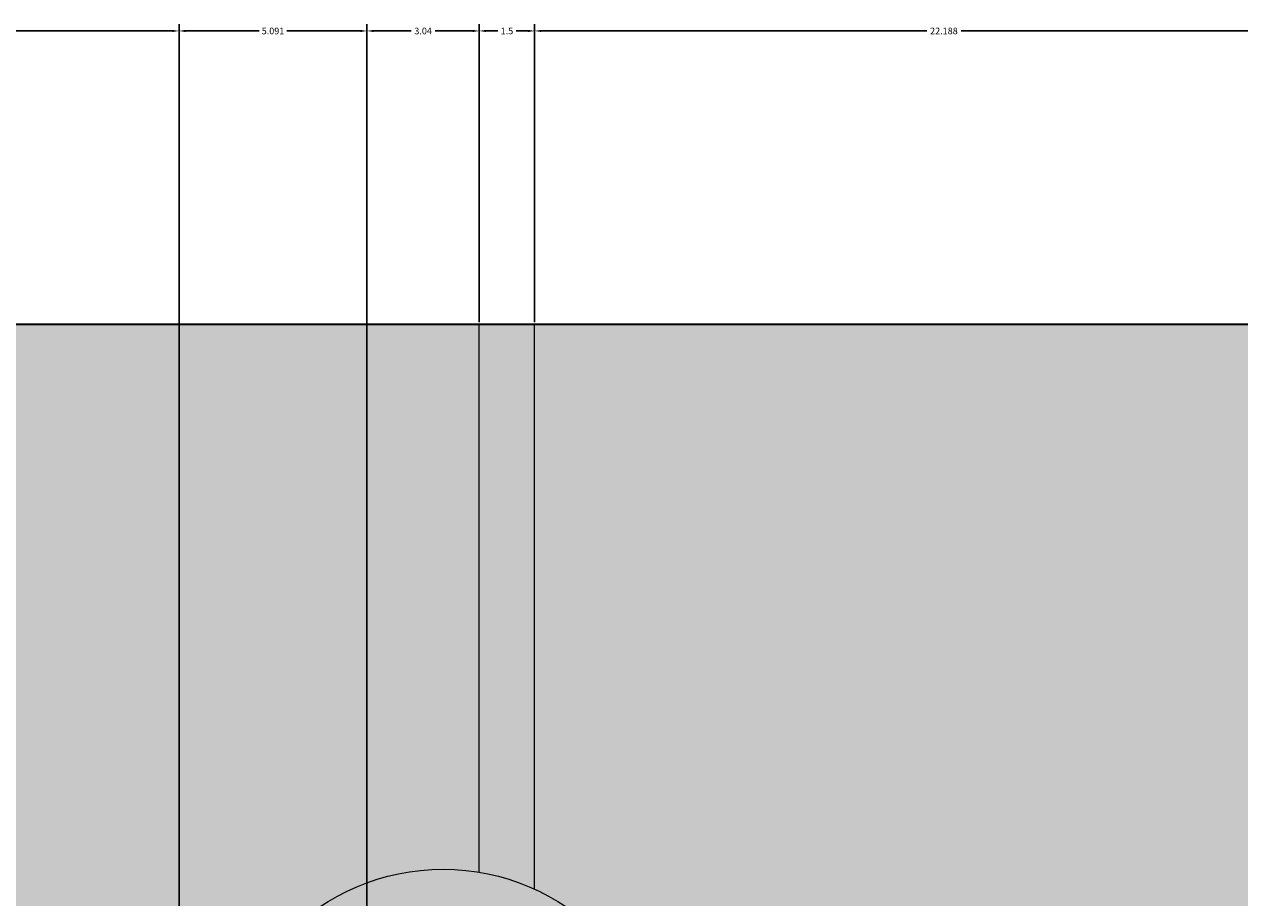
# Model space of a CAD drawing. Units: inches. Extents: x 4508 to 4723, y 847 to 1020.
# Tile 30 of 32: x 4658 to 4691, y 979 to 1003. Entities that reach past the tile are written whole.
import ezdxf

# ---------------------------------------------------------------- set-up
doc = ezdxf.new("R2010")
doc.units = ezdxf.units.IN
for name, color, linetype, lineweight in [('A-ANNO-DIMS', 2, 'Continuous', 18), ('A-WALL', 7, 'Continuous', 35), ('A-WALL-DECO', 6, 'Continuous', 18), ('A-WALL-PATT', 254, 'Continuous', 13)]:
    doc.layers.add(name, color=color, linetype=linetype, lineweight=lineweight)
doc.styles.get("Standard").update_dxf_attribs({"font": 'arial.ttf'})
doc.dimstyles.get("Standard").update_dxf_attribs({"dimtxt": 0.18, "dimasz": 0.18, "dimexe": 0.18, "dimexo": 0.0625, "dimgap": 0.09, "dimtad": 0, "dimtih": 1, "dimtoh": 1, "dimdec": 4, "dimzin": 0, "dimdsep": 46, "dimtxsty": 'Standard', "dimcen": 0.09, "dimadec": 0, "dimazin": 0, "dimtfac": 1, "dimtdec": 4, "dimtofl": 0, "dimtmove": 0, "dimatfit": 3, "dimfxl": 1, "dimtolj": 1, "dimtzin": 0, "dimarcsym": 0})

# ---------------------------------------------------------------- blocks, each defined once
blk = doc.blocks.new('*D7')
at = {"layer": 'A-ANNO-DIMS', "color": 0, "lineweight": -2, "transparency": 16777216}
for p, q in [((4588.994, 994.809), (4588.994, 1002.877)), ((4662.171, 957.665), (4662.171, 1002.877)), ((4589.174, 1002.697), (4625.189, 1002.697)), ((4661.991, 1002.697), (4625.975, 1002.697))]:
    blk.add_line(p, q, dxfattribs=at)
at = {"layer": 'A-ANNO-DIMS', "color": 0, "lineweight": 9, "transparency": 16777216}
for points in [[(4589.174, 1002.727), (4589.174, 1002.667), (4588.994, 1002.697)], [(4661.991, 1002.727), (4661.991, 1002.667), (4662.171, 1002.697)]]:
    blk.add_solid(points, dxfattribs=at)
at = {"layer": 'Defpoints', "color": 0, "lineweight": 9, "transparency": 16777216}
for p in [(4662.171, 1002.697), (4588.994, 994.747), (4662.171, 957.602)]:
    blk.add_point(p, dxfattribs=at)
at = {"layer": 'A-ANNO-DIMS', "color": 0, "transparency": 16777216, "insert": (4625.582, 1002.697), "char_height": 0.18, "attachment_point": 5}
blk.add_mtext('\\A1;73.18', dxfattribs=at)
blk = doc.blocks.new('*D8')
at = {"layer": 'A-ANNO-DIMS', "color": 0, "lineweight": -2, "transparency": 16777216}
for p, q in [((4662.171, 957.665), (4662.171, 1002.877)), ((4667.262, 936.184), (4667.262, 1002.877)), ((4662.351, 1002.697), (4664.34, 1002.697)), ((4667.082, 1002.697), (4665.092, 1002.697))]:
    blk.add_line(p, q, dxfattribs=at)
at = {"layer": 'A-ANNO-DIMS', "color": 0, "lineweight": 9, "transparency": 16777216}
for points in [[(4662.351, 1002.727), (4662.351, 1002.667), (4662.171, 1002.697)], [(4667.082, 1002.727), (4667.082, 1002.667), (4667.262, 1002.697)]]:
    blk.add_solid(points, dxfattribs=at)
at = {"layer": 'Defpoints', "color": 0, "lineweight": 9, "transparency": 16777216}
for p in [(4667.262, 1002.697), (4662.171, 957.602), (4667.262, 936.122)]:
    blk.add_point(p, dxfattribs=at)
at = {"layer": 'A-ANNO-DIMS', "color": 0, "transparency": 16777216, "insert": (4664.716, 1002.697), "char_height": 0.18, "attachment_point": 5}
blk.add_mtext('\\A1;5.091', dxfattribs=at)
blk = doc.blocks.new('*D9')
at = {"layer": 'A-ANNO-DIMS', "color": 0, "lineweight": -2, "transparency": 16777216}
for p, q in [((4667.262, 936.184), (4667.262, 1002.877)), ((4670.306, 994.809), (4670.306, 1002.877)), ((4667.442, 1002.697), (4668.461, 1002.697)), ((4670.126, 1002.697), (4669.107, 1002.697))]:
    blk.add_line(p, q, dxfattribs=at)
at = {"layer": 'A-ANNO-DIMS', "color": 0, "lineweight": 9, "transparency": 16777216}
for points in [[(4667.442, 1002.727), (4667.442, 1002.667), (4667.262, 1002.697)], [(4670.126, 1002.727), (4670.126, 1002.667), (4670.306, 1002.697)]]:
    blk.add_solid(points, dxfattribs=at)
at = {"layer": 'Defpoints', "color": 0, "lineweight": 9, "transparency": 16777216}
for p in [(4670.306, 1002.697), (4670.306, 994.747), (4667.262, 936.122)]:
    blk.add_point(p, dxfattribs=at)
at = {"layer": 'A-ANNO-DIMS', "color": 0, "transparency": 16777216, "insert": (4668.784, 1002.697), "char_height": 0.18, "attachment_point": 5}
blk.add_mtext('\\A1;3.04', dxfattribs=at)
blk = doc.blocks.new('*D10')
at = {"layer": 'A-ANNO-DIMS', "color": 0, "lineweight": -2, "transparency": 16777216}
for p, q in [((4670.306, 994.809), (4670.306, 1002.877)), ((4671.806, 994.809), (4671.806, 1002.877)), ((4670.486, 1002.697), (4670.81, 1002.697)), ((4671.626, 1002.697), (4671.302, 1002.697))]:
    blk.add_line(p, q, dxfattribs=at)
at = {"layer": 'A-ANNO-DIMS', "color": 0, "lineweight": 9, "transparency": 16777216}
for points in [[(4670.486, 1002.727), (4670.486, 1002.667), (4670.306, 1002.697)], [(4671.626, 1002.727), (4671.626, 1002.667), (4671.806, 1002.697)]]:
    blk.add_solid(points, dxfattribs=at)
at = {"layer": 'Defpoints', "color": 0, "lineweight": 9, "transparency": 16777216}
for p in [(4671.806, 1002.697), (4670.306, 994.747), (4671.806, 994.747)]:
    blk.add_point(p, dxfattribs=at)
at = {"layer": 'A-ANNO-DIMS', "color": 0, "transparency": 16777216, "insert": (4671.056, 1002.697), "char_height": 0.18, "attachment_point": 5}
blk.add_mtext('\\A1;1.5', dxfattribs=at)
blk = doc.blocks.new('*D11')
at = {"layer": 'A-ANNO-DIMS', "color": 0, "lineweight": -2, "transparency": 16777216}
for p, q in [((4671.806, 994.809), (4671.806, 1002.877)), ((4693.994, 994.809), (4693.994, 1002.877)), ((4671.986, 1002.697), (4682.435, 1002.697)), ((4693.814, 1002.697), (4683.365, 1002.697))]:
    blk.add_line(p, q, dxfattribs=at)
at = {"layer": 'A-ANNO-DIMS', "color": 0, "lineweight": 9, "transparency": 16777216}
for points in [[(4671.986, 1002.727), (4671.986, 1002.667), (4671.806, 1002.697)], [(4693.814, 1002.727), (4693.814, 1002.667), (4693.994, 1002.697)]]:
    blk.add_solid(points, dxfattribs=at)
at = {"layer": 'Defpoints', "color": 0, "lineweight": 9, "transparency": 16777216}
for p in [(4693.994, 1002.697), (4671.806, 994.747), (4693.994, 994.747)]:
    blk.add_point(p, dxfattribs=at)
at = {"layer": 'A-ANNO-DIMS', "color": 0, "transparency": 16777216, "insert": (4682.9, 1002.697), "char_height": 0.18, "attachment_point": 5}
blk.add_mtext('\\A1;22.188', dxfattribs=at)
blk = doc.blocks.new('*D23')
at = {"layer": 'A-ANNO-DIMS', "color": 0, "lineweight": -2, "transparency": 16777216}
for p, q in [((4694.056, 994.747), (4702.124, 994.747)), ((4701.944, 994.567), (4701.944, 984.545)), ((4701.944, 974.158), (4701.944, 984.181)), ((4669.387, 973.978), (4702.124, 973.978))]:
    blk.add_line(p, q, dxfattribs=at)
at = {"layer": 'A-ANNO-DIMS', "color": 0, "lineweight": 9, "transparency": 16777216}
for points in [[(4701.914, 994.567), (4701.974, 994.567), (4701.944, 994.747)], [(4701.914, 974.158), (4701.974, 974.158), (4701.944, 973.978)]]:
    blk.add_solid(points, dxfattribs=at)
at = {"layer": 'Defpoints', "color": 0, "lineweight": 9, "transparency": 16777216}
for p in [(4693.994, 994.747), (4701.944, 994.747), (4669.325, 973.978)]:
    blk.add_point(p, dxfattribs=at)
at = {"layer": 'A-ANNO-DIMS', "color": 0, "transparency": 16777216, "insert": (4701.944, 984.363), "char_height": 0.18, "attachment_point": 5}
blk.add_mtext('\\A1;20.77', dxfattribs=at)

msp = doc.modelspace()

# ---------------------------------------------------------------- hatches: boundary and pattern name
at = {"layer": 'A-WALL-PATT', "transparency": 33554508}
h = msp.add_hatch(color=256, dxfattribs=at)
h.dxf.hatch_style = 1
h.paths.add_polyline_path([(4661.6706, 954.043, -0.3739004), (4658.5765, 957.6021, -1), (4665.7646, 957.6021, -0.3739004), (4662.6706, 954.043), (4662.6706, 944.4021, -0.2114781), (4670.3062, 945.0869), (4670.3062, 968.0592, -0.4632086), (4663.3246, 973.9783, -0.4632086), (4670.3062, 979.8975), (4670.3062, 994.7469), (4588.9938, 994.7469), (4588.9938, 904.7469), (4657.9938, 904.7469), (4657.9938, 886.7469), (4549.9938, 886.7469), (4549.9938, 878.7469), (4693.9938, 878.7469), (4693.9938, 994.7469), (4671.8062, 994.7469), (4671.8062, 979.4411, -0.2941682), (4675.3246, 973.9783, -0.2941682), (4671.8062, 968.5156), (4671.8062, 944.4278, -0.2741114), (4676.7298, 936.1217, -0.2741114), (4671.8062, 927.8155), (4671.8062, 907.6998, -0.3779645), (4677.0562, 901.7469, -0.3779645), (4671.8062, 895.7939), (4671.8062, 883.7469), (4670.3062, 883.7469), (4670.3062, 895.7939, -0.3779645), (4665.0562, 901.7469, -0.3779645), (4670.3062, 907.6998), (4670.3062, 927.1564, -0.2114781), (4662.6706, 927.8412), (4662.6706, 918.2003, -0.3739004), (4665.7646, 914.6412, -1), (4658.5765, 914.6412, -0.3739004), (4661.6706, 918.2003), (4661.6706, 928.4807, -0.2391825), (4657.7936, 936.1217, -0.2391825), (4661.6706, 943.7626)])
at = {"layer": 'A-WALL-PATT', "transparency": 33554681}
h = msp.add_hatch(color=256, dxfattribs=at)
h.dxf.hatch_style = 1
h.paths.add_polyline_path([(4671.8062, 968.5156, -0.0656104), (4670.3062, 968.0592), (4670.3062, 945.0869, -0.0433429), (4671.8062, 944.4278)])
h.paths.add_polyline_path([(4662.6706, 954.043, -0.0698991), (4661.6706, 954.043), (4661.6706, 943.7626, -0.0313734), (4662.6706, 944.4021)])
h.paths.add_polyline_path([(4665.7646, 957.6021, 1), (4658.5765, 957.6021, 1)])
h.paths.add_polyline_path([(4659.0765, 957.6021, -1), (4665.2646, 957.6021, -1)], flags=16)
h.paths.add_polyline_path([(4675.3246, 973.9783, 1), (4663.3246, 973.9783, 1)])
h.paths.add_polyline_path([(4664.3246, 973.9783, -1), (4674.3246, 973.9783, -1)], flags=16)
h.paths.add_polyline_path([(4671.8062, 994.7469), (4670.3062, 994.7469), (4670.3062, 979.8975, -0.0656104), (4671.8062, 979.4411)])

# ---------------------------------------------------------------- linework, layer by layer
at = {"layer": 'A-WALL'}
msp.add_line((4540.9938, 994.7469), (4693.9938, 994.7469), dxfattribs=at)
at = {"layer": 'A-WALL-DECO'}
for p, q in [((4670.3062, 979.8975), (4670.3062, 994.7469)), ((4671.8062, 979.4411), (4671.8062, 994.7469))]:
    msp.add_line(p, q, dxfattribs=at)
msp.add_circle((4669.3246, 973.9783), 6, dxfattribs=at)

# ---------------------------------------------------------------- dimensions: what is measured, and where the dimension line sits
at = {"layer": 'A-ANNO-DIMS'}
for base, p1, p2, override, picture, middle in [((4662.1706, 1002.6969), (4588.9938, 994.7469), (4662.1706, 957.6021), {"dimdec": 2, "dimlfac": 1, "dimrnd": 0, "dimzin": 0, "dimdsep": 46, "dimlunit": 2}, '*D7', (4625.5822, 1002.6969)), ((4667.2617, 1002.6969), (4662.1706, 957.6021), (4667.2617, 936.1217), {"dimdec": 3, "dimlfac": 1, "dimrnd": 0, "dimzin": 0, "dimdsep": 46, "dimlunit": 2}, '*D8', (4664.7161, 1002.6969)), ((4670.3062, 1002.6969), (4667.2617, 936.1217), (4670.3062, 994.7469), {"dimdec": 2, "dimlfac": 1, "dimrnd": 0, "dimzin": 0, "dimdsep": 46, "dimlunit": 2}, '*D9', (4668.7839, 1002.6969)), ((4671.8062, 1002.6969), (4670.3062, 994.7469), (4671.8062, 994.7469), {"dimdec": 1, "dimlfac": 1, "dimrnd": 0, "dimzin": 0, "dimdsep": 46, "dimlunit": 2}, '*D10', (4671.0562, 1002.6969)), ((4693.9938, 1002.6969), (4671.8062, 994.7469), (4693.9938, 994.7469), {"dimdec": 3, "dimlfac": 1, "dimrnd": 0, "dimzin": 0, "dimdsep": 46, "dimlunit": 2}, '*D11', (4682.9, 1002.6969))]:
    dim = msp.add_linear_dim(base=base, p1=p1, p2=p2, dimstyle='Standard', override=override, dxfattribs=at)
    dim.commit()
    dim.dimension.update_dxf_attribs({"geometry": picture, "text_midpoint": middle})
dim = msp.add_linear_dim(base=(4701.9438, 994.7469), p1=(4669.3246, 973.9783), p2=(4693.9938, 994.7469), angle=90, dimstyle='Standard', override={"dimdec": 2, "dimlfac": 1, "dimrnd": 0, "dimzin": 0, "dimdsep": 46, "dimlunit": 2}, dxfattribs=at)
dim.commit()
dim.dimension.update_dxf_attribs({"geometry": '*D23', "text_midpoint": (4701.9438, 984.3626)})

doc.saveas('drawing.dxf')
